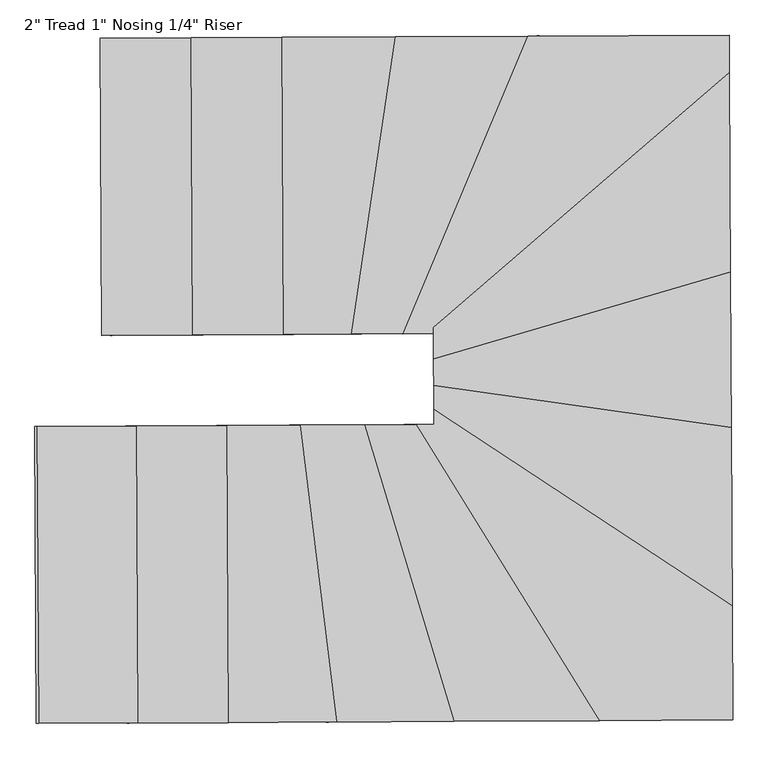
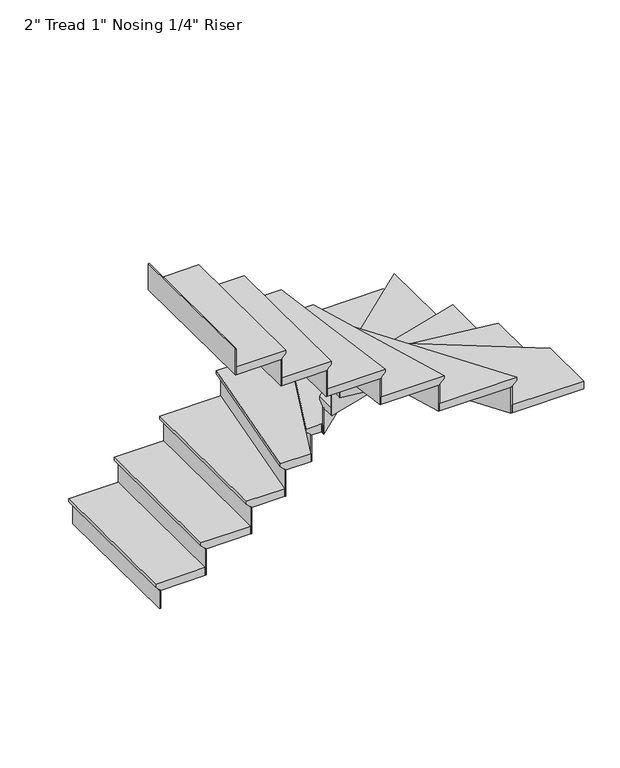
"""IFC4 building model written with IfcOpenShell, lengths in millimetres: stair flight geometry."""

from ifc_helpers import new_model, si_unit, origin, place, context, project, spatial, faceted_brep, source, transform, mapped, element, save


def stair_flight_456e8720(model_context):
    return source(origin(), model_context, "Body", "Brep", [
        faceted_brep([(73.5214139, -4197.1296428, 3858.6833333), (73.5214139, -4197.1296428, 3877.7333333), (68.8012135, -3282.7418259, 3877.7333333), (68.8012135, -3282.7418259, 3858.6833333), (98.9210755, -4196.9985261, 3833.2833333), (94.200875, -3282.6107092, 3833.2833333), (378.3173529, -4195.5562427, 3877.7333333), (373.5971524, -3281.1684258, 3877.7333333), (94.200875, -3282.6107092, 3826.9333333), (373.5971524, -3281.1684258, 3826.9333333), (378.3173529, -4195.5562427, 3826.9333333), (98.9210755, -4196.9985261, 3826.9333333)], [[[0, 1, 2, 3]], [[4, 0, 3, 5]], [[2, 1, 6, 7]], [[8, 9, 10, 11]], [[2, 7, 9, 8, 5, 3]], [[8, 11, 4, 5]], [[6, 1, 0, 4, 11, 10]], [[7, 6, 10, 9]]]),
        faceted_brep([(98.9210755, -4196.9985261, 3826.9333333), (98.9210755, -4196.9985261, 3708.4), (105.2709909, -4196.965747, 3708.4), (105.2709909, -4196.965747, 3826.9333333), (94.200875, -3282.6107092, 3826.9333333), (100.5507904, -3282.5779301, 3826.9333333), (100.5507904, -3282.5779301, 3708.4), (94.200875, -3282.6107092, 3708.4)], [[[0, 1, 2, 3]], [[4, 5, 6, 7]], [[1, 0, 4, 7]], [[2, 1, 7, 6]], [[3, 2, 6, 5]], [[0, 3, 5, 4]]]),
        faceted_brep([(378.3173529, -4195.5562427, 3996.2666667), (378.3173529, -4195.5562427, 3826.9333333), (384.6672683, -4195.5234635, 3826.9333333), (384.6672683, -4195.5234635, 3996.2666667), (373.5971524, -3281.1684258, 3996.2666667), (379.9470678, -3281.1356466, 3996.2666667), (379.9470678, -3281.1356466, 3826.9333333), (373.5971524, -3281.1684258, 3826.9333333)], [[[0, 1, 2, 3]], [[4, 5, 6, 7]], [[1, 0, 4, 7]], [[2, 1, 7, 6]], [[3, 2, 6, 5]], [[0, 3, 5, 4]]]),
        faceted_brep([(348.1974909, -3281.2995425, 4047.0666667), (352.9176913, -4195.6873594, 4047.0666667), (657.7136303, -4194.1139592, 4047.0666667), (652.9934298, -3279.7261423, 4047.0666667), (373.5971524, -3281.1684258, 3996.2666667), (652.9934298, -3279.7261423, 3996.2666667), (657.7136303, -4194.1139592, 3996.2666667), (378.3173529, -4195.5562427, 3996.2666667), (373.5971524, -3281.1684258, 4002.6166667), (348.1974909, -3281.2995425, 4028.0166667), (378.3173529, -4195.5562427, 4002.6166667), (352.9176913, -4195.6873594, 4028.0166667)], [[[0, 1, 2, 3]], [[4, 5, 6, 7]], [[0, 3, 5, 4, 8, 9]], [[4, 7, 10, 8]], [[2, 1, 11, 10, 7, 6]], [[3, 2, 6, 5]], [[11, 1, 0, 9]], [[10, 11, 9, 8]]]),
        faceted_brep([(657.7136303, -4194.1139592, 4165.6), (657.7136303, -4194.1139592, 3996.2666667), (664.0635457, -4194.08118, 3996.2666667), (664.0635457, -4194.08118, 4165.6), (652.9934298, -3279.7261423, 4165.6), (659.3433452, -3279.6933631, 4165.6), (659.3433452, -3279.6933631, 3996.2666667), (652.9934298, -3279.7261423, 3996.2666667)], [[[0, 1, 2, 3]], [[4, 5, 6, 7]], [[1, 0, 4, 7]], [[2, 1, 7, 6]], [[3, 2, 6, 5]], [[0, 3, 5, 4]]]),
        faceted_brep([(627.5937682, -3279.857259, 4216.4), (632.3139687, -4194.2450759, 4216.4), (866.9504995, -4193.0338486, 4216.4), (1003.1488336, -3277.9185901, 4216.4), (652.9934298, -3279.7261423, 4165.6), (1003.1488336, -3277.9185901, 4165.6), (866.9504995, -4193.0338486, 4165.6), (657.7136303, -4194.1139592, 4165.6), (652.9934298, -3279.7261423, 4171.95), (627.5937682, -3279.857259, 4197.35), (657.7136303, -4194.1139592, 4171.95), (632.3139687, -4194.2450759, 4197.35)], [[[0, 1, 2, 3]], [[4, 5, 6, 7]], [[0, 3, 5, 4, 8, 9]], [[4, 7, 10, 8]], [[2, 1, 11, 10, 7, 6]], [[3, 2, 6, 5]], [[11, 1, 0, 9]], [[10, 11, 9, 8]]]),
        faceted_brep([(866.9504995, -4193.0338486, 4334.9333333), (866.9504995, -4193.0338486, 4165.6), (873.3753797, -4193.0006825, 4165.6), (873.3753797, -4193.0006825, 4334.9333333), (1003.1488336, -3277.9185901, 4334.9333333), (1009.5737138, -3277.885424, 4334.9333333), (1009.5737138, -3277.885424, 4165.6), (1003.1488336, -3277.9185901, 4165.6)], [[[0, 1, 2, 3]], [[4, 5, 6, 7]], [[1, 0, 4, 7]], [[2, 1, 7, 6]], [[3, 2, 6, 5]], [[0, 3, 5, 4]]]),
        faceted_brep([(977.4493129, -3278.0512547, 4385.7333333), (841.2509788, -4193.1665132, 4385.7333333), (1028.3454494, -4192.2007049, 4385.7333333), (1412.7936505, -3275.8039451, 4385.7333333), (1003.1488336, -3277.9185901, 4334.9333333), (1412.7936505, -3275.8039451, 4334.9333333), (1028.3454494, -4192.2007049, 4334.9333333), (866.9504995, -4193.0338486, 4334.9333333), (1003.1488336, -3277.9185901, 4341.2833333), (977.4493129, -3278.0512547, 4366.6833333), (866.9504995, -4193.0338486, 4341.2833333), (841.2509788, -4193.1665132, 4366.6833333)], [[[0, 1, 2, 3]], [[4, 5, 6, 7]], [[0, 3, 5, 4, 8, 9]], [[4, 7, 10, 8]], [[2, 1, 11, 10, 7, 6]], [[3, 2, 6, 5]], [[11, 1, 0, 9]], [[10, 11, 9, 8]]]),
        faceted_brep([(1028.3454494, -4192.2007049, 4504.2666667), (1028.3454494, -4192.2007049, 4334.9333333), (1035.2465542, -4192.1650804, 4334.9333333), (1035.2465542, -4192.1650804, 4504.2666667), (1412.7936505, -3275.8039451, 4504.2666667), (1419.6947553, -3275.7683206, 4504.2666667), (1419.6947553, -3275.7683206, 4334.9333333), (1412.7936505, -3275.8039451, 4334.9333333)], [[[0, 1, 2, 3]], [[4, 5, 6, 7]], [[1, 0, 4, 7]], [[2, 1, 7, 6]], [[3, 2, 6, 5]], [[0, 3, 5, 4]]]),
        faceted_brep([(2004.5597861, -3422.5660243, 4555.0666667), (2003.7864306, -3272.753156, 4555.0666667), (1385.1892314, -3275.9464431, 4555.0666667), (1000.7410303, -4192.3432028, 4555.0666667), (1094.1188142, -4191.8611734, 4555.0666667), (1094.1970217, -4207.0113762, 4555.0666667), (2003.7864306, -3272.753156, 4504.2666667), (2004.5597861, -3422.5660243, 4504.2666667), (1094.1970217, -4207.0113762, 4504.2666667), (1094.1188142, -4191.8611734, 4504.2666667), (1028.3454494, -4192.2007049, 4504.2666667), (1412.7936505, -3275.8039451, 4504.2666667), (1028.3454494, -4192.2007049, 4510.6166667), (1412.7936505, -3275.8039451, 4510.6166667), (1000.7410303, -4192.3432028, 4536.0166667), (1385.1892314, -3275.9464431, 4536.0166667)], [[[0, 1, 2, 3, 4, 5]], [[6, 7, 8, 9, 10, 11]], [[1, 0, 7, 6]], [[11, 10, 12, 13]], [[4, 3, 14, 12, 10, 9]], [[0, 5, 8, 7]], [[14, 3, 2, 15]], [[12, 14, 15, 13]], [[2, 1, 6, 11, 13, 15]], [[5, 4, 9, 8]]]),
        faceted_brep([(1094.1970217, -4207.0113762, 4673.6), (1094.1970217, -4207.0113762, 4504.2666667), (1094.2401004, -4215.3564963, 4504.2666667), (1094.2401004, -4215.3564963, 4673.6), (2004.5597861, -3422.5660243, 4673.6), (2004.6028648, -3430.9111444, 4673.6), (2004.6028648, -3430.9111444, 4504.2666667), (2004.5597861, -3422.5660243, 4504.2666667)], [[[0, 1, 2, 3]], [[4, 5, 6, 7]], [[1, 0, 4, 7]], [[2, 1, 7, 6]], [[3, 2, 6, 5]], [[0, 3, 5, 4]]]),
        faceted_brep([(2004.3874713, -3389.1855438, 4724.4), (1094.0247069, -4173.6308957, 4724.4), (1094.654759, -4295.6833292, 4724.4), (2007.6910705, -4029.1522065, 4724.4), (2004.5597861, -3422.5660243, 4673.6), (2007.6910705, -4029.1522065, 4673.6), (1094.654759, -4295.6833292, 4673.6), (1094.1970217, -4207.0113762, 4673.6), (2004.5597861, -3422.5660243, 4679.95), (2004.3874713, -3389.1855438, 4705.35), (1094.1970217, -4207.0113762, 4679.95), (1094.0247069, -4173.6308957, 4705.35)], [[[0, 1, 2, 3]], [[4, 5, 6, 7]], [[0, 3, 5, 4, 8, 9]], [[4, 7, 10, 8]], [[3, 2, 6, 5]], [[11, 1, 0, 9]], [[10, 11, 9, 8]], [[2, 1, 11, 10, 7, 6]]]),
        faceted_brep([(1094.654759, -4295.6833292, 4842.9333333), (1094.654759, -4295.6833292, 4673.6), (1094.6888553, -4302.2884051, 4673.6), (1094.6888553, -4302.2884051, 4842.9333333), (2007.6910705, -4029.1522065, 4842.9333333), (2007.7251669, -4035.7572823, 4842.9333333), (2007.7251669, -4035.7572823, 4673.6), (2007.6910705, -4029.1522065, 4673.6)], [[[0, 1, 2, 3]], [[4, 5, 6, 7]], [[1, 0, 4, 7]], [[2, 1, 7, 6]], [[3, 2, 6, 5]], [[0, 3, 5, 4]]]),
        faceted_brep([(2007.5546851, -4002.7319029, 4893.7333333), (1094.5183736, -4269.2630257, 4893.7333333), (1095.0784269, -4377.7554326, 4893.7333333), (2010.1530082, -4506.0738629, 4893.7333333), (2007.6910705, -4029.1522065, 4842.9333333), (2010.1530082, -4506.0738629, 4842.9333333), (1095.0784269, -4377.7554326, 4842.9333333), (1094.654759, -4295.6833292, 4842.9333333), (2007.6910705, -4029.1522065, 4849.2833333), (2007.5546851, -4002.7319029, 4874.6833333), (1094.654759, -4295.6833292, 4849.2833333), (1094.5183736, -4269.2630257, 4874.6833333)], [[[0, 1, 2, 3]], [[4, 5, 6, 7]], [[0, 3, 5, 4, 8, 9]], [[4, 7, 10, 8]], [[2, 1, 11, 10, 7, 6]], [[3, 2, 6, 5]], [[11, 1, 0, 9]], [[10, 11, 9, 8]]]),
        faceted_brep([(1095.0784269, -4377.7554326, 5012.2666667), (1095.0784269, -4377.7554326, 4842.9333333), (1095.1115512, -4384.1722058, 4842.9333333), (1095.1115512, -4384.1722058, 5012.2666667), (2010.1530082, -4506.0738629, 5012.2666667), (2010.1861325, -4512.4906361, 5012.2666667), (2010.1861325, -4512.4906361, 4842.9333333), (2010.1530082, -4506.0738629, 4842.9333333)], [[[0, 1, 2, 3]], [[4, 5, 6, 7]], [[1, 0, 4, 7]], [[2, 1, 7, 6]], [[3, 2, 6, 5]], [[0, 3, 5, 4]]]),
        faceted_brep([(2010.020511, -4480.40677, 5063.0666667), (1094.9459297, -4352.0883397, 5063.0666667), (1095.4823291, -4455.9985745, 5063.0666667), (2013.0146854, -5060.4322638, 5063.0666667), (2010.1530082, -4506.0738629, 5012.2666667), (2013.0146854, -5060.4322638, 5012.2666667), (1095.4823291, -4455.9985745, 5012.2666667), (1095.0784269, -4377.7554326, 5012.2666667), (2010.1530082, -4506.0738629, 5018.6166667), (2010.020511, -4480.40677, 5044.0166667), (1095.0784269, -4377.7554326, 5018.6166667), (1094.9459297, -4352.0883397, 5044.0166667)], [[[0, 1, 2, 3]], [[4, 5, 6, 7]], [[0, 3, 5, 4, 8, 9]], [[4, 7, 10, 8]], [[3, 2, 6, 5]], [[11, 1, 0, 9]], [[10, 11, 9, 8]], [[2, 1, 11, 10, 7, 6]]]),
        faceted_brep([(1095.4823291, -4455.9985745, 5181.6), (1095.4823291, -4455.9985745, 5012.2666667), (1095.5217161, -4463.6285363, 5012.2666667), (1095.5217161, -4463.6285363, 5181.6), (2013.0146854, -5060.4322638, 5181.6), (2013.0540723, -5068.0622255, 5181.6), (2013.0540723, -5068.0622255, 5012.2666667), (2013.0146854, -5060.4322638, 5012.2666667)], [[[0, 1, 2, 3]], [[4, 5, 6, 7]], [[1, 0, 4, 7]], [[2, 1, 7, 6]], [[3, 2, 6, 5]], [[0, 3, 5, 4]]]),
        faceted_brep([(1574.7396622, -5383.1960459, 5232.4), (2014.669115, -5380.9250672, 5232.4), (2012.8571376, -5029.9124167, 5232.4), (1095.3247813, -4425.4787274, 5232.4), (1095.5610976, -4471.2574507, 5232.4), (1010.2079956, -4471.6980556, 5232.4), (2014.669115, -5380.9250672, 5181.6), (1574.7396622, -5383.1960459, 5181.6), (1010.2079956, -4471.6980556, 5181.6), (1095.5610976, -4471.2574507, 5181.6), (1095.4823291, -4455.9985745, 5181.6), (2013.0146854, -5060.4322638, 5181.6), (1095.4823291, -4455.9985745, 5187.95), (2013.0146854, -5060.4322638, 5187.95), (1095.3247813, -4425.4787274, 5213.35), (2012.8571376, -5029.9124167, 5213.35)], [[[0, 1, 2, 3, 4, 5]], [[6, 7, 8, 9, 10, 11]], [[1, 0, 7, 6]], [[11, 10, 12, 13]], [[4, 3, 14, 12, 10, 9]], [[0, 5, 8, 7]], [[14, 3, 2, 15]], [[12, 14, 15, 13]], [[5, 4, 9, 8]], [[2, 1, 6, 11, 13, 15]]]),
        faceted_brep([(1010.2079956, -4471.6980556, 5350.9333333), (1010.2079956, -4471.6980556, 5181.6), (1002.7625472, -4471.7364901, 5181.6), (1002.7625472, -4471.7364901, 5350.9333333), (1574.7396622, -5383.1960459, 5350.9333333), (1567.2942139, -5383.2344803, 5350.9333333), (1567.2942139, -5383.2344803, 5181.6), (1574.7396622, -5383.1960459, 5181.6)], [[[0, 1, 2, 3]], [[4, 5, 6, 7]], [[1, 0, 4, 7]], [[2, 1, 7, 6]], [[3, 2, 6, 5]], [[0, 3, 5, 4]]]),
        faceted_brep([(1604.5214555, -5383.042308, 5401.7333333), (1039.9897889, -4471.5443178, 5401.7333333), (854.9585932, -4472.4994752, 5401.7333333), (1130.3137603, -5385.4902358, 5401.7333333), (1574.7396622, -5383.1960459, 5350.9333333), (1130.3137603, -5385.4902358, 5350.9333333), (854.9585932, -4472.4994752, 5350.9333333), (1010.2079956, -4471.6980556, 5350.9333333), (1574.7396622, -5383.1960459, 5357.2833333), (1604.5214555, -5383.042308, 5382.6833333), (1010.2079956, -4471.6980556, 5357.2833333), (1039.9897889, -4471.5443178, 5382.6833333)], [[[0, 1, 2, 3]], [[4, 5, 6, 7]], [[0, 3, 5, 4, 8, 9]], [[4, 7, 10, 8]], [[2, 1, 11, 10, 7, 6]], [[3, 2, 6, 5]], [[11, 1, 0, 9]], [[10, 11, 9, 8]]]),
        faceted_brep([(854.9585932, -4472.4994752, 5520.2666667), (854.9585932, -4472.4994752, 5350.9333333), (848.3363877, -4472.53366, 5350.9333333), (848.3363877, -4472.53366, 5520.2666667), (1130.3137603, -5385.4902358, 5520.2666667), (1123.6915548, -5385.5244206, 5520.2666667), (1123.6915548, -5385.5244206, 5350.9333333), (1130.3137603, -5385.4902358, 5350.9333333)], [[[0, 1, 2, 3]], [[4, 5, 6, 7]], [[1, 0, 4, 7]], [[2, 1, 7, 6]], [[3, 2, 6, 5]], [[0, 3, 5, 4]]]),
        faceted_brep([(1156.8025822, -5385.3534967, 5571.0666667), (881.4474152, -4472.3627361, 5571.0666667), (657.851655, -4473.5169694, 5571.0666667), (770.454123, -5387.3478826, 5571.0666667), (1130.3137603, -5385.4902358, 5520.2666667), (770.454123, -5387.3478826, 5520.2666667), (657.851655, -4473.5169694, 5520.2666667), (854.9585932, -4472.4994752, 5520.2666667), (1130.3137603, -5385.4902358, 5526.6166667), (1156.8025822, -5385.3534967, 5552.0166667), (854.9585932, -4472.4994752, 5526.6166667), (881.4474152, -4472.3627361, 5552.0166667)], [[[0, 1, 2, 3]], [[4, 5, 6, 7]], [[0, 3, 5, 4, 8, 9]], [[4, 7, 10, 8]], [[2, 1, 11, 10, 7, 6]], [[3, 2, 6, 5]], [[11, 1, 0, 9]], [[10, 11, 9, 8]]]),
        faceted_brep([(657.851655, -4473.5169694, 5689.6), (657.851655, -4473.5169694, 5520.2666667), (651.457697, -4473.5499759, 5520.2666667), (651.457697, -4473.5499759, 5689.6), (770.454123, -5387.3478826, 5689.6), (764.060165, -5387.3808891, 5689.6), (764.060165, -5387.3808891, 5520.2666667), (770.454123, -5387.3478826, 5520.2666667)], [[[0, 1, 2, 3]], [[4, 5, 6, 7]], [[1, 0, 4, 7]], [[2, 1, 7, 6]], [[3, 2, 6, 5]], [[0, 3, 5, 4]]]),
        faceted_brep([(796.0299553, -5387.2158565, 5740.4), (683.4274873, -4473.3849433, 5740.4), (432.5726821, -4474.6798916, 5740.4), (437.2928826, -5389.0677085, 5740.4), (770.454123, -5387.3478826, 5689.6), (437.2928826, -5389.0677085, 5689.6), (432.5726821, -4474.6798916, 5689.6), (657.851655, -4473.5169694, 5689.6), (770.454123, -5387.3478826, 5695.95), (796.0299553, -5387.2158565, 5721.35), (657.851655, -4473.5169694, 5695.95), (683.4274873, -4473.3849433, 5721.35)], [[[0, 1, 2, 3]], [[4, 5, 6, 7]], [[0, 3, 5, 4, 8, 9]], [[4, 7, 10, 8]], [[2, 1, 11, 10, 7, 6]], [[3, 2, 6, 5]], [[11, 1, 0, 9]], [[10, 11, 9, 8]]]),
        faceted_brep([(432.5726821, -4474.6798916, 5858.9333333), (432.5726821, -4474.6798916, 5689.6), (426.2227667, -4474.7126708, 5689.6), (426.2227667, -4474.7126708, 5858.9333333), (437.2928826, -5389.0677085, 5858.9333333), (430.9429672, -5389.1004877, 5858.9333333), (430.9429672, -5389.1004877, 5689.6), (437.2928826, -5389.0677085, 5689.6)], [[[0, 1, 2, 3]], [[4, 5, 6, 7]], [[1, 0, 4, 7]], [[2, 1, 7, 6]], [[3, 2, 6, 5]], [[0, 3, 5, 4]]]),
        faceted_brep([(462.6925441, -5388.9365918, 5909.7333333), (457.9723437, -4474.5487749, 5909.7333333), (153.1764047, -4476.1221751, 5909.7333333), (157.8966052, -5390.509992, 5909.7333333), (437.2928826, -5389.0677085, 5858.9333333), (157.8966052, -5390.509992, 5858.9333333), (153.1764047, -4476.1221751, 5858.9333333), (432.5726821, -4474.6798916, 5858.9333333), (437.2928826, -5389.0677085, 5865.2833333), (462.6925441, -5388.9365918, 5890.6833333), (432.5726821, -4474.6798916, 5865.2833333), (457.9723437, -4474.5487749, 5890.6833333)], [[[0, 1, 2, 3]], [[4, 5, 6, 7]], [[0, 3, 5, 4, 8, 9]], [[4, 7, 10, 8]], [[2, 1, 11, 10, 7, 6]], [[3, 2, 6, 5]], [[11, 1, 0, 9]], [[10, 11, 9, 8]]]),
        faceted_brep([(153.1764047, -4476.1221751, 6028.2666667), (153.1764047, -4476.1221751, 5858.9333333), (146.8264893, -4476.1549542, 5858.9333333), (146.8264893, -4476.1549542, 6028.2666667), (157.8966052, -5390.509992, 6028.2666667), (151.5466898, -5390.5427711, 6028.2666667), (151.5466898, -5390.5427711, 5858.9333333), (157.8966052, -5390.509992, 5858.9333333)], [[[0, 1, 2, 3]], [[4, 5, 6, 7]], [[1, 0, 4, 7]], [[2, 1, 7, 6]], [[3, 2, 6, 5]], [[0, 3, 5, 4]]]),
        faceted_brep([(-126.2198726, -4477.5644585, 6197.6), (-126.2198726, -4477.5644585, 6028.2666667), (-132.569788, -4477.5972377, 6028.2666667), (-132.569788, -4477.5972377, 6197.6), (-121.4996722, -5391.9522754, 6197.6), (-127.8495876, -5391.9850546, 6197.6), (-127.8495876, -5391.9850546, 6028.2666667), (-121.4996722, -5391.9522754, 6028.2666667)], [[[0, 1, 2, 3]], [[4, 5, 6, 7]], [[1, 0, 4, 7]], [[2, 1, 7, 6]], [[3, 2, 6, 5]], [[0, 3, 5, 4]]]),
        faceted_brep([(183.2962668, -5390.3788753, 6079.0666667), (178.5760663, -4475.9910584, 6079.0666667), (-126.2198726, -4477.5644585, 6079.0666667), (-121.4996722, -5391.9522754, 6079.0666667), (157.8966052, -5390.509992, 6028.2666667), (-121.4996722, -5391.9522754, 6028.2666667), (-126.2198726, -4477.5644585, 6028.2666667), (153.1764047, -4476.1221751, 6028.2666667), (157.8966052, -5390.509992, 6034.6166667), (183.2962668, -5390.3788753, 6060.0166667), (153.1764047, -4476.1221751, 6034.6166667), (178.5760663, -4475.9910584, 6060.0166667)], [[[0, 1, 2, 3]], [[4, 5, 6, 7]], [[0, 3, 5, 4, 8, 9]], [[4, 7, 10, 8]], [[2, 1, 11, 10, 7, 6]], [[3, 2, 6, 5]], [[11, 1, 0, 9]], [[10, 11, 9, 8]]]),
    ])


if __name__ == "__main__":
    model = new_model("IFC4")
    model_context = context("Model", 3, world=origin())
    ifc_project = project(units=[si_unit("LENGTHUNIT", "METRE", prefix="MILLI")], contexts=[model_context])
    site = spatial("IfcSite", under=ifc_project)
    building = spatial("IfcBuilding", under=site)
    placement = place(None, origin())
    stair_flight_shape = stair_flight_456e8720(model_context)
    element("IfcStairFlight", 1, ObjectType="2\" Tread 1\" Nosing 1/4\" Riser", at=placement, inside=building, context=model_context, shape_type="MappedRepresentation", body=[
        mapped(stair_flight_shape, transform((0.0, 0.0, 0.0), x_axis=(1.0, 0.0, 0.0), y_axis=(0.0, 1.0, 0.0), z_axis=(0.0, 0.0, 1.0))),
    ])
    save(model, "model.ifc")
